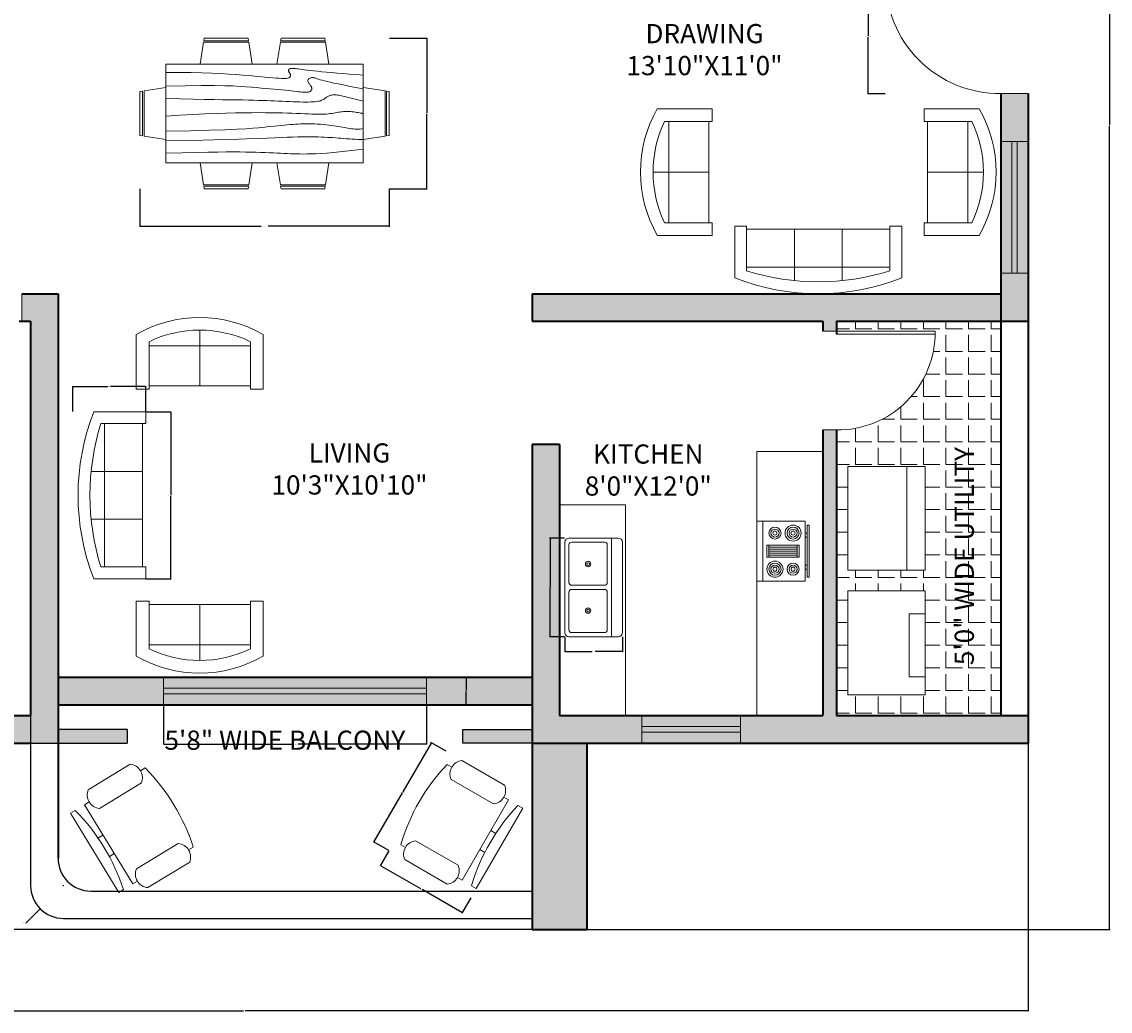
# Model space of a CAD drawing. Units: inches. Extents: x -382 to 250, y 518 to 1732.
# Tile 2 of 8: x -147 to 250, y 518 to 879. Entities that reach past the tile are written whole.
import ezdxf

# ---------------------------------------------------------------- set-up
doc = ezdxf.new("R2010")
doc.units = ezdxf.units.IN
doc.header["$MEASUREMENT"] = 0
for name, color, linetype, lineweight in [('A-ANNO-DIMS', 2, 'Continuous', 18), ('A-AREA-IDEN', 7, 'Continuous', 18), ('A-DOOR', 3, 'Continuous', 18), ('A-EQPM', 9, 'Continuous', 18), ('A-FLOR-CASE', 8, 'Continuous', 18), ('A-FLOR-EDGE', 7, 'Continuous', 25), ('A-FLOR-FIXT', 8, 'Continuous', 18), ('A-FLOR-PATT', 9, 'Continuous', 13), ('A-FURN', 8, 'Continuous', 18), ('A-GLAZ', 4, 'Continuous', 18), ('A-WALL', 7, 'Continuous', 35)]:
    doc.layers.add(name, color=color, linetype=linetype, lineweight=lineweight)
doc.layers.add('A-GLAZ-PATT', color=143, linetype='Continuous', lineweight=13, true_color=0x7aafdf)
doc.layers.add('A-WALL-PATT', color=251, linetype='Continuous', lineweight=13, true_color=0x636466)
doc.styles.get("Standard").update_dxf_attribs({"font": 'arial.ttf'})
doc.dimstyles.get("Standard").update_dxf_attribs({"dimtxt": 0.18, "dimasz": 0.18, "dimexe": 0.18, "dimexo": 0.0625, "dimgap": 0.09, "dimtad": 0, "dimtih": 1, "dimtoh": 1, "dimdec": 4, "dimzin": 0, "dimdsep": 46, "dimtxsty": 'Standard', "dimcen": 0.09, "dimadec": 0, "dimazin": 0, "dimtfac": 1, "dimtdec": 4, "dimtofl": 0, "dimtmove": 0, "dimatfit": 3, "dimfxl": 1, "dimtolj": 1, "dimtzin": 0, "dimarcsym": 0})

# ---------------------------------------------------------------- blocks, each defined once
blk = doc.blocks.new('Dining Set - 36 x 72 in.')
for p, q in [((-22.2343, 26.00059), (-23.4847, 17.99762)), ((-22.2304, 26), (-5.7608, 26)), ((-22, 27.5), (-22.1562, 26.50042)), ((-5.8416, 26.5), (-22.1534, 26.5)), ((-22, 27.5), (-6, 27.5)), ((-5.8437, 26.49966), (-6, 27.5)), ((-4.5152, 17.99762), (-5.7655, 25.99926)), ((5.7657, 26.00059), (4.5153, 17.99762)), ((5.7696, 26), (22.2392, 26)), ((6, 27.5), (5.8438, 26.50042)), ((22.1584, 26.5), (5.8466, 26.5)), ((6, 27.5), (22, 27.5)), ((22.1563, 26.49966), (22, 27.5)), ((23.4848, 17.99762), (22.2345, 25.99926)), ((36, 18), (-36, 18)), ((-36, 18), (-36, -18)), ((36, -18), (36, 18)), ((-45.5, 8), (-44.5004, 8.15617)), ((-45.5, 8), (-45.5, -8)), ((-44.5, -8.15843), (-44.5, 8.15338)), ((-44.0006, 8.23428), (-35.9976, 9.48474)), ((-44, 8.23041), (-44, -8.23915)), ((44.0006, 8.23428), (35.9976, 9.48474)), ((44, 8.23041), (44, -8.23915)), ((44.5, -8.15843), (44.5, 8.15338)), ((45.5, 8), (44.5005, 8.15617)), ((45.5, 8), (45.5, -8)), ((-44.4997, -8.15631), (-45.5, -8)), ((-35.9976, -9.48476), (-43.9993, -8.2345)), ((35.9976, -9.48476), (43.9993, -8.2345)), ((44.4997, -8.15631), (45.5, -8)), ((-36, -18), (36, -18)), ((-22.2343, -26.0006), (-23.4847, -17.99762)), ((-4.5152, -17.99762), (-5.7655, -25.99928)), ((5.7657, -26.0006), (4.5153, -17.99762)), ((23.4848, -17.99762), (22.2345, -25.99928)), ((-22.2304, -26), (-5.7608, -26)), ((-22, -27.5), (-22.1562, -26.50044)), ((-5.8416, -26.5), (-22.1534, -26.5)), ((-22, -27.5), (-6, -27.5)), ((-5.8437, -26.49967), (-6, -27.5)), ((5.7696, -26), (22.2392, -26)), ((6, -27.5), (5.8438, -26.50044)), ((22.1584, -26.5), (5.8466, -26.5)), ((6, -27.5), (22, -27.5)), ((22.1563, -26.49967), (22, -27.5))]:
    blk.add_line(p, q)
for points in [[(-36, 15), (-31.1772, 14.97754), (-26.8079, 14.91406), (-22.8538, 14.81543), (-19.276, 14.6875), (-16.0362, 14.53613), (-13.0957, 14.36718), (-10.4159, 14.18652), (-7.9583, 14), (-5.6904, 13.81315), (-3.6035, 13.63021), (-1.6954, 13.45508), (0.0365, 13.29166), (1.5945, 13.14388), (2.9811, 13.01562), (4.1988, 12.9108), (5.25, 12.83333), (6.1393, 12.78613), (6.8802, 12.76823), (7.4883, 12.77767), (7.9792, 12.8125), (8.3685, 12.87077), (8.6719, 12.95052), (8.9049, 13.0498), (9.0833, 13.16666), (9.2205, 13.29899), (9.3216, 13.44401), (9.3895, 13.59879), (9.4271, 13.76041), (9.4373, 13.92594), (9.4232, 14.09245), (9.3875, 14.257), (9.3333, 14.41666), (9.2638, 14.56917), (9.1836, 14.71484), (9.0975, 14.85465), (9.0104, 14.98958), (8.9272, 15.1206), (8.8529, 15.2487), (8.7922, 15.37483), (8.75, 15.5), (8.7305, 15.62467), (8.7344, 15.74739), (8.7617, 15.86621), (8.8125, 15.97916), (8.8867, 16.08431), (8.9844, 16.17968), (9.1055, 16.26334), (9.25, 16.33333), (9.4189, 16.38802), (9.6172, 16.42708), (9.8506, 16.45052), (10.125, 16.45833), (10.4463, 16.45052), (10.8203, 16.42708), (11.2529, 16.38802), (11.75, 16.33333), (12.3184, 16.26318), (12.9694, 16.17838), (13.7151, 16.07991), (14.5677, 15.96875), (15.5395, 15.84586), (16.6426, 15.71224), (17.8893, 15.56884), (19.2917, 15.41666), (20.859, 15.25667), (22.5879, 15.08984), (24.4721, 14.91715), (26.5052, 14.73958), (28.6809, 14.5581), (30.9929, 14.3737), (33.4347, 14.18733), (36, 14)], [(-36, 10), (-28.9766, 10.14274), (-23.1725, 10.20442), (-18.4241, 10.19775), (-14.5677, 10.13541), (-11.4399, 10.03011), (-8.877, 9.89453), (-6.7154, 9.74137), (-4.7917, 9.58333), (-2.9698, 9.43082), (-1.2246, 9.28515), (0.4415, 9.14534), (2.026, 9.01041), (3.5266, 8.87939), (4.9408, 8.7513), (6.266, 8.62516), (7.5, 8.5), (8.6411, 8.37549), (9.6914, 8.2539), (10.6538, 8.13818), (11.5312, 8.03125), (12.3267, 7.93603), (13.043, 7.85547), (13.6831, 7.79248), (14.25, 7.75), (14.7471, 7.7303), (15.1797, 7.73307), (15.5537, 7.75732), (15.875, 7.80208), (16.1494, 7.86637), (16.3828, 7.94922), (16.5811, 8.04964), (16.75, 8.16666), (16.8944, 8.29915), (17.0143, 8.44531), (17.1089, 8.60319), (17.1771, 8.77083), (17.218, 8.94629), (17.2305, 9.1276), (17.2137, 9.31282), (17.1667, 9.5), (17.0895, 9.6875), (16.987, 9.875), (16.8649, 10.0625), (16.7292, 10.25), (16.5856, 10.4375), (16.4401, 10.625), (16.2985, 10.8125), (16.1667, 11), (16.05, 11.18733), (15.9518, 11.3737), (15.8752, 11.5581), (15.8229, 11.73958), (15.798, 11.91715), (15.8034, 12.08984), (15.842, 12.25667), (15.9167, 12.41666), (16.0295, 12.56836), (16.1784, 12.70833), (16.3605, 12.83268), (16.5729, 12.9375), (16.8127, 13.01888), (17.0768, 13.07291), (17.3625, 13.0957), (17.6667, 13.08333), (17.9894, 13.03312), (18.3418, 12.94726), (18.7382, 12.82918), (19.1927, 12.68229), (19.7195, 12.51001), (20.3327, 12.31575), (21.0465, 12.10294), (21.875, 11.875), (22.8357, 11.63354), (23.959, 11.37304), (25.2786, 11.08618), (26.8282, 10.76562), (28.6414, 10.40405), (30.752, 9.99414), (33.1936, 9.52856), (36, 9)], [(-36, 5.5), (-30.7157, 5.3348), (-26.069, 5.20963), (-21.9946, 5.11767), (-18.4271, 5.05208), (-15.3009, 5.00602), (-12.5508, 4.97265), (-10.1112, 4.94515), (-7.9167, 4.91666), (-5.909, 4.88167), (-4.0586, 4.83984), (-2.3429, 4.79215), (-0.7396, 4.73958), (0.7739, 4.6831), (2.22, 4.6237), (3.6213, 4.56233), (5, 4.5), (6.373, 4.43782), (7.7344, 4.3776), (9.0723, 4.32129), (10.375, 4.27083), (11.6309, 4.22819), (12.8281, 4.19531), (13.9551, 4.17415), (15, 4.16666), (15.954, 4.17448), (16.819, 4.19791), (17.6001, 4.23698), (18.3021, 4.29166), (18.9299, 4.36198), (19.4883, 4.44791), (19.9823, 4.54948), (20.4167, 4.66666), (20.7969, 4.79899), (21.1302, 4.94401), (21.4245, 5.09879), (21.6875, 5.26041), (21.9271, 5.42594), (22.1511, 5.59245), (22.3672, 5.757), (22.5834, 5.91666), (22.8065, 6.06868), (23.0404, 6.21093), (23.2879, 6.34147), (23.5521, 6.45833), (23.8358, 6.55957), (24.142, 6.64323), (24.4735, 6.70735), (24.8334, 6.75), (25.2235, 6.76969), (25.642, 6.76692), (26.0858, 6.74267), (26.5521, 6.69791), (27.0379, 6.63362), (27.5404, 6.55078), (28.0565, 6.45036), (28.5834, 6.33333), (29.1242, 6.19987), (29.7071, 6.04687), (30.3661, 5.87044), (31.1354, 5.66666), (32.0493, 5.43164), (33.142, 5.16146), (34.4475, 4.85221), (36, 4.5)], [(-36, -1), (-30.7915, -0.6591), (-26.0195, -0.38216), (-21.6519, -0.16284), (-17.6563, 0.00521), (-14.0005, 0.12833), (-10.6523, 0.21289), (-7.5796, 0.26522), (-4.75, 0.29166), (-2.134, 0.29793), (0.2878, 0.28711), (2.5317, 0.26163), (4.6146, 0.22396), (6.5529, 0.17651), (8.3633, 0.12174), (10.0623, 0.06209), (11.6667, 0), (13.1899, -0.06201), (14.6341, -0.1211), (15.9982, -0.17432), (17.2813, -0.21875), (18.4823, -0.25147), (19.6003, -0.26953), (20.6343, -0.27002), (21.5834, -0.25), (22.4481, -0.20768), (23.2357, -0.14584), (23.9549, -0.06836), (24.6146, 0.02083), (25.2235, 0.11784), (25.7904, 0.21875), (26.3241, 0.31966), (26.8334, 0.41666), (27.3265, 0.50618), (27.8099, 0.58593), (28.2894, 0.65397), (28.7709, 0.70833), (29.2601, 0.74707), (29.763, 0.76823), (30.2855, 0.76985), (30.8334, 0.75), (31.4088, 0.70784), (31.9994, 0.64713), (32.589, 0.57275), (33.1615, 0.48958), (33.7008, 0.4025), (34.1908, 0.3164), (34.6153, 0.23616), (34.9584, 0.16666), (35.2099, 0.11165), (35.3848, 0.07031), (35.504, 0.04069), (35.5886, 0.02083), (35.6594, 0.00879), (35.7377, 0.0026), (35.8442, 0.00032), (36, 0)], [(-36, -6.5), (-27.1843, -6.31267), (-20.084, -6.1263), (-14.469, -5.9419), (-10.1094, -5.76042), (-6.7752, -5.58285), (-4.2363, -5.41016), (-2.2629, -5.24333), (-0.625, -5.08334), (0.8708, -4.93099), (2.2715, -4.78646), (3.5872, -4.64974), (4.8281, -4.52084), (6.0046, -4.39974), (7.127, -4.28646), (8.2053, -4.18099), (9.25, -4.08334), (10.2705, -3.99382), (11.2734, -3.91407), (12.2647, -3.84603), (13.25, -3.79167), (14.2354, -3.75293), (15.2266, -3.73177), (16.2295, -3.73015), (17.25, -3.75), (18.2912, -3.79248), (19.3451, -3.85547), (20.4009, -3.93604), (21.4479, -4.03125), (22.4754, -4.13819), (23.4727, -4.25391), (24.4289, -4.37549), (25.3334, -4.5), (26.1785, -4.62492), (26.9694, -4.74935), (27.7145, -4.87281), (28.4219, -4.99479), (29.1, -5.11483), (29.7572, -5.23242), (30.4016, -5.34709), (31.0417, -5.45834), (31.6837, -5.56437), (32.3262, -5.65821), (32.9658, -5.73153), (33.599, -5.77604), (34.2224, -5.78345), (34.8327, -5.74545), (35.4264, -5.65373), (36, -5.5)], [(-36, -10), (-26.4022, -9.81299), (-18.4675, -9.62891), (-11.9839, -9.45069), (-6.7396, -9.28125), (-2.5226, -9.12354), (0.8789, -8.98047), (3.6769, -8.85498), (6.0833, -8.75), (8.2767, -8.66765), (10.3021, -8.60677), (12.1712, -8.56543), (13.8958, -8.54167), (15.4876, -8.53353), (16.9583, -8.53907), (18.3197, -8.55632), (19.5834, -8.58334), (20.7616, -8.61841), (21.8685, -8.66081), (22.9188, -8.71004), (23.9271, -8.76563), (24.9081, -8.82707), (25.8763, -8.89388), (26.8465, -8.96558), (27.8334, -9.04167), (28.8474, -9.12118), (29.8828, -9.20117), (30.93, -9.27824), (31.9792, -9.34896), (33.0205, -9.40991), (34.0443, -9.45768), (35.0407, -9.48885), (36, -9.5)], [(-36, -14.5), (-30.0881, -14.33513), (-25.0332, -14.21224), (-20.7312, -14.12647), (-17.0781, -14.07292), (-13.97, -14.04671), (-11.3027, -14.04297), (-8.9724, -14.05681), (-6.875, -14.08334), (-4.9224, -14.11833), (-3.0905, -14.16016), (-1.3709, -14.20785), (0.2448, -14.26042), (1.7647, -14.3169), (3.1973, -14.3763), (4.5507, -14.43767), (5.8333, -14.5), (7.0554, -14.5621), (8.235, -14.62175), (9.3922, -14.67652), (10.5469, -14.72396), (11.7192, -14.76164), (12.929, -14.78711), (14.1965, -14.79794), (15.5417, -14.79167), (16.9933, -14.76424), (18.6152, -14.70508), (20.4804, -14.60197), (22.6615, -14.44271), (25.2312, -14.21509), (28.2624, -13.9069), (31.8277, -13.50594), (36, -13)]]:
    blk.add_lwpolyline(points)
blk = doc.blocks.new('Chair - Desk')
for p, q in [((-8.5, 0), (-8.5, -1)), ((-8.5, 0), (8.5, 0)), ((8.5, 0), (8.5, -1)), ((-2, -3), (-2, -1.9355)), ((2, -1.9576), (2, -3)), ((-8.5, -3), (-8.5, -4)), ((-8.5, -3), (8.5, -3)), ((8.5, -3), (8.5, -4)), ((-10.5, -5), (-10.5, -14)), ((-6.5, -14), (-6.5, -5)), ((6.5, -5), (6.5, -14)), ((10.5, -14), (10.5, -5)), ((-8.5, -15), (-8.5, -16)), ((8.5, -15), (8.5, -16))]:
    blk.add_line(p, q)
for centre, radius, start, end in [((0, 34.625), 36.625, 256.5803, 283.4197), ((-8.5, -6.5), 2.5, 36.8699, 143.1301), ((8.5, -6.5), 2.5, 36.8699, 143.1301), ((-8.5, -12.5), 2.5, 216.8699, 323.1301), ((8.5, -12.5), 2.5, 216.8699, 323.1301), ((0, 19.625), 36.625, 256.5803, 283.4197)]:
    blk.add_arc(centre, radius, start, end)
blk = doc.blocks.new('Sofa - Roundback 7 ft.')
for p, q in [((-12.00002, -32.4421), (-12.00003, -6.5971)), ((11.99997, -32.4421), (11.99998, -6.5971)), ((-36.000027, -34), (-36.000027, -11.4696)), ((-35.999844, -13.3819), (35.9998, -13.3819)), ((35.99998, -34), (35.99998, -11.4696)), ((-36.000027, -32.4421), (35.99998, -32.4421))]:
    blk.add_line(p, q)
for points in [[(-36.000027, -34), (-42.000027, -34), (-42.000027, -8)], [(41.99998, -8), (41.99998, -34), (35.99998, -34)]]:
    blk.add_lwpolyline(points)
for centre, radius, start, end in [((0, -114.25), 114.25, 68.43141, 111.5686), ((-0.00001, -127.1968), 121.1968, 72.72033, 107.2797)]:
    blk.add_arc(centre, radius, start, end)
blk = doc.blocks.new('Sofa - Roundback Loveseat 5 ft.')
for p, q in [((0, -32.44198), (0, -5.99998)), ((-24, -33.99998), (-24, -11.46958)), ((-23.9998, -13.38178), (23.99986, -13.38178)), ((24.00004, -33.99998), (24.00004, -11.46958)), ((-24, -32.44198), (24.00004, -32.44198))]:
    blk.add_line(p, q)
for points in [[(-24, -33.99998), (-30, -33.99998), (-30, -7.99998)], [(30.00004, -7.99998), (30.00004, -33.99998), (24.00004, -33.99998)]]:
    blk.add_lwpolyline(points)
for centre, radius, start, end in [((0, -60.24998), 60.24998, 60.13715, 119.8628), ((0, -61.38438), 55.38444, 64.32083, 115.6792)]:
    blk.add_arc(centre, radius, start, end)
blk = doc.blocks.new('Sink-double - 36 in top')
for p, q in [((-18, -4), (18, -4)), ((-0.75, -18.5), (-0.75, -6.5)), ((0.75, -6.5), (0.75, -18.5))]:
    blk.add_line(p, q)
for points in [[(-16.5, 0), (16.5, 0)], [(-18, -19.5), (-18, -1.5)], [(18, -1.5), (18, -19.5)], [(-16.5, -18.5), (-16.5, -6.5)], [(-15.5, -5.5), (-1.75, -5.5)], [(1.75, -5.5), (15.5, -5.5)], [(16.5, -6.5), (16.5, -18.5)], [(-1.75, -19.5), (-15.5, -19.5)], [(15.5, -19.5), (1.75, -19.5)], [(16.5, -21), (-16.5, -21)]]:
    blk.add_lwpolyline(points)
for centre, radius in [((-8.5, -12.5), 1), ((8.5, -12.5), 1), ((-8.5, -12.5), 0.5), ((8.5, -12.5), 0.5)]:
    blk.add_circle(centre, radius)
for centre, radius, start, end in [((-16.5, -1.5), 1.5, 90, 180), ((16.5, -1.5), 1.5, 0, 90), ((-15.5, -6.5), 1, 90, 180), ((-1.75, -6.5), 1, 0, 90), ((1.75, -6.5), 1, 90, 180), ((15.5, -6.5), 1, 0, 90), ((-16.5, -19.5), 1.5, 180, 270), ((-15.5, -18.5), 1, 180, 270), ((-1.75, -18.5), 1, 270, 0), ((1.75, -18.5), 1, 180, 270), ((15.5, -18.5), 1, 270, 0), ((16.5, -19.5), 1.5, 270, 0)]:
    blk.add_arc(centre, radius, start, end)
blk = doc.blocks.new('Range-Oven - 30 in top')
for p, q in [((0, -3), (30, -3)), ((12, -6), (18, -6)), ((13, -20), (13, -6)), ((14, -6), (14, -20)), ((15, -20), (15, -6)), ((16, -6), (16, -20)), ((17, -20), (17, -6)), ((18, -20), (12, -20)), ((6, -24), (6, -25)), ((8, -25), (8, -24)), ((22, -25), (22, -24)), ((24, -24), (24, -25))]:
    blk.add_line(p, q)
for points in [[(0, -24), (0, 0), (30, 0), (30, -24)], [(12, -21), (12, -5), (18, -5), (18, -21)], [(2, -26), (2, -25), (28, -25), (28, -26)]]:
    blk.add_lwpolyline(points, close=True)
for centre, radius in [((6, -9), 4), ((6, -9), 3), ((6, -9), 2), ((6, -9), 1), ((24, -9), 3), ((24, -9), 2), ((24, -9), 1), ((6, -18), 3), ((6, -18), 2), ((24, -18), 4), ((24, -18), 3), ((24, -18), 2), ((6, -18), 1), ((24, -18), 1)]:
    blk.add_circle(centre, radius)
blk = doc.blocks.new('DOOR-SWING-36IN')
for p, q in [((-1, 0), (-1, 36)), ((0, 0), (0, 36))]:
    blk.add_line(p, q)
blk.add_arc((-0.5, 0.5), 35.5, 89.1931, 180.8069)
blk = doc.blocks.new('GLAZ-BALCONY-96IN')
for p, q in [((0, 10), (0, 0)), ((96, 10), (96, 0)), ((0, 6), (96, 6)), ((0, 4), (96, 4))]:
    blk.add_line(p, q)
blk = doc.blocks.new('DOOR-ENTRY-42IN')
for p, q in [((0, 0), (-42, 0)), ((0, -1), (-42, -1))]:
    blk.add_line(p, q)
blk.add_arc((-0.5, -0.5), 41.5, 179.3097, 270.6903)
blk = doc.blocks.new('*D34')
at = {"layer": 'A-ANNO-DIMS', "color": 0, "lineweight": -2, "transparency": 16777216}
for p, q in [((-102.16, 736.99), (-92.9, 736.99)), ((-93.08, 736.81), (-93.08, 706.68)), ((-93.08, 676.19), (-93.08, 706.32)), ((-102.16, 676.01), (-92.9, 676.01))]:
    blk.add_line(p, q, dxfattribs=at)
at = {"layer": 'A-ANNO-DIMS', "color": 0, "transparency": 16777216}
for points in [[(-93.11, 736.81), (-93.05, 736.81), (-93.08, 736.99)], [(-93.11, 676.19), (-93.05, 676.19), (-93.08, 676.01)]]:
    blk.add_solid(points, dxfattribs=at)
at = {"layer": 'Defpoints', "color": 0, "transparency": 16777216}
for p in [(-102.23, 736.99), (-93.08, 736.99), (-102.23, 676.01)]:
    blk.add_point(p, dxfattribs=at)
at = {"layer": 'A-ANNO-DIMS', "color": 0, "transparency": 16777216, "insert": (-93.08, 706.5), "char_height": 0.18, "attachment_point": 5}
blk.add_mtext('\\A1;SOFA 61 TYP.', dxfattribs=at)
blk = doc.blocks.new('*D35')
at = {"layer": 'A-ANNO-DIMS', "color": 0, "lineweight": -2, "transparency": 16777216}
for p, q in [((-128.84, 737.05), (-128.84, 746.32)), ((-128.66, 746.14), (-116.06, 746.14)), ((-102.41, 746.14), (-115.01, 746.14)), ((-102.23, 737.05), (-102.23, 746.32))]:
    blk.add_line(p, q, dxfattribs=at)
at = {"layer": 'A-ANNO-DIMS', "color": 0, "transparency": 16777216}
for points in [[(-128.66, 746.17), (-128.66, 746.11), (-128.84, 746.14)], [(-102.41, 746.17), (-102.41, 746.11), (-102.23, 746.14)]]:
    blk.add_solid(points, dxfattribs=at)
at = {"layer": 'Defpoints', "color": 0, "transparency": 16777216}
for p in [(-128.84, 746.14), (-128.84, 736.99), (-102.23, 736.99)]:
    blk.add_point(p, dxfattribs=at)
at = {"layer": 'A-ANNO-DIMS', "color": 0, "transparency": 16777216, "insert": (-115.54, 746.14), "char_height": 0.18, "attachment_point": 5}
blk.add_mtext('\\A1;27 TYP.', dxfattribs=at)
blk = doc.blocks.new('*D36')
at = {"layer": 'A-ANNO-DIMS', "color": 0, "lineweight": -2, "transparency": 16777216}
for p, q in [((1.91, 616.01), (-8.35, 598.25)), ((7.37, 613.06), (1.84, 616.26)), ((-18.82, 580.12), (-8.56, 597.88)), ((-13.53, 576.86), (-19.06, 580.05))]:
    blk.add_line(p, q, dxfattribs=at)
at = {"layer": 'A-ANNO-DIMS', "color": 0, "transparency": 16777216}
for points in [[(1.88, 616.02), (1.93, 615.99), (2, 616.17)], [(-18.84, 580.13), (-18.79, 580.1), (-18.91, 579.96)]]:
    blk.add_solid(points, dxfattribs=at)
at = {"layer": 'Defpoints', "color": 0, "transparency": 16777216}
for p in [(7.43, 613.03), (-18.91, 579.96), (-13.48, 576.83)]:
    blk.add_point(p, dxfattribs=at)
at = {"layer": 'A-ANNO-DIMS', "color": 0, "transparency": 16777216, "insert": (-8.46, 598.06), "char_height": 0.18, "attachment_point": 5}
blk.add_mtext('\\A1;CHAIR 42 TYP.', dxfattribs=at)
blk = doc.blocks.new('*D37')
at = {"layer": 'A-ANNO-DIMS', "color": 0, "lineweight": -2, "transparency": 16777216}
for p, q in [((-13.51, 576.77), (-16.7, 571.24)), ((-16.46, 571.31), (-1.99, 562.95)), ((13.12, 554.23), (-1.36, 562.59)), ((16.38, 559.52), (13.18, 553.99))]:
    blk.add_line(p, q, dxfattribs=at)
at = {"layer": 'A-ANNO-DIMS', "color": 0, "transparency": 16777216}
for points in [[(-16.44, 571.33), (-16.47, 571.28), (-16.61, 571.4)], [(13.13, 554.26), (13.1, 554.21), (13.27, 554.14)]]:
    blk.add_solid(points, dxfattribs=at)
at = {"layer": 'Defpoints', "color": 0, "transparency": 16777216}
for p in [(-13.48, 576.83), (16.41, 559.57), (13.27, 554.14)]:
    blk.add_point(p, dxfattribs=at)
at = {"layer": 'A-ANNO-DIMS', "color": 0, "transparency": 16777216, "insert": (-1.67, 562.77), "char_height": 0.18, "attachment_point": 5}
blk.add_mtext('\\A1;35 TYP.', dxfattribs=at)
blk = doc.blocks.new('*D40')
at = {"layer": 'A-ANNO-DIMS', "color": 0, "lineweight": -2, "transparency": 16777216}
for p, q in [((-104.34, 818.28), (-104.34, 804.52)), ((-13.34, 818.28), (-13.34, 804.52)), ((-104.16, 804.7), (-60.12, 804.7)), ((-13.52, 804.7), (-57.56, 804.7))]:
    blk.add_line(p, q, dxfattribs=at)
at = {"layer": 'A-ANNO-DIMS', "color": 0, "transparency": 16777216}
for points in [[(-104.16, 804.73), (-104.16, 804.67), (-104.34, 804.7)], [(-13.52, 804.73), (-13.52, 804.67), (-13.34, 804.7)]]:
    blk.add_solid(points, dxfattribs=at)
at = {"layer": 'Defpoints', "color": 0, "transparency": 16777216}
for p in [(-104.34, 818.35), (-13.34, 818.35), (-13.34, 804.7)]:
    blk.add_point(p, dxfattribs=at)
at = {"layer": 'A-ANNO-DIMS', "color": 0, "transparency": 16777216, "insert": (-58.84, 804.7), "char_height": 0.18, "attachment_point": 5}
blk.add_mtext('\\A1;DINING SET 91 TYP.', dxfattribs=at)
blk = doc.blocks.new('*D41')
at = {"layer": 'A-ANNO-DIMS', "color": 0, "lineweight": -2, "transparency": 16777216}
for p, q in [((-13.28, 873.35), (0.49, 873.35)), ((0.31, 873.17), (0.31, 846.03)), ((0.31, 818.53), (0.31, 845.66)), ((-13.28, 818.35), (0.49, 818.35))]:
    blk.add_line(p, q, dxfattribs=at)
at = {"layer": 'A-ANNO-DIMS', "color": 0, "transparency": 16777216}
for points in [[(0.28, 873.17), (0.34, 873.17), (0.31, 873.35)], [(0.28, 818.53), (0.34, 818.53), (0.31, 818.35)]]:
    blk.add_solid(points, dxfattribs=at)
at = {"layer": 'Defpoints', "color": 0, "transparency": 16777216}
for p in [(-13.34, 873.35), (0.31, 873.35), (-13.34, 818.35)]:
    blk.add_point(p, dxfattribs=at)
at = {"layer": 'A-ANNO-DIMS', "color": 0, "transparency": 16777216, "insert": (0.31, 845.85), "char_height": 0.18, "attachment_point": 5}
blk.add_mtext('\\A1;55 TYP.', dxfattribs=at)
blk = doc.blocks.new('*D46')
at = {"layer": 'A-ANNO-DIMS', "color": 0, "lineweight": -2, "transparency": 16777216}
for p, q in [((50.64, 690.89), (45.12, 690.89)), ((45.3, 690.71), (45.3, 673.08)), ((45.3, 655.07), (45.3, 672.71)), ((50.64, 654.89), (45.12, 654.89))]:
    blk.add_line(p, q, dxfattribs=at)
at = {"layer": 'A-ANNO-DIMS', "color": 0, "transparency": 16777216}
for points in [[(45.27, 690.71), (45.33, 690.71), (45.3, 690.89)], [(45.27, 655.07), (45.33, 655.07), (45.3, 654.89)]]:
    blk.add_solid(points, dxfattribs=at)
at = {"layer": 'Defpoints', "color": 0, "transparency": 16777216}
for p in [(50.7, 690.89), (45.3, 654.89), (50.7, 654.89)]:
    blk.add_point(p, dxfattribs=at)
at = {"layer": 'A-ANNO-DIMS', "color": 0, "transparency": 16777216, "insert": (45.3, 672.89), "char_height": 0.18, "attachment_point": 5}
blk.add_mtext('\\A1;SINK 36 TYP.', dxfattribs=at)
blk = doc.blocks.new('*D47')
at = {"layer": 'A-ANNO-DIMS', "color": 0, "lineweight": -2, "transparency": 16777216}
for p, q in [((50.7, 654.83), (50.7, 649.31)), ((71.7, 654.83), (71.7, 649.31)), ((50.88, 649.49), (60.67, 649.49)), ((71.52, 649.49), (61.73, 649.49))]:
    blk.add_line(p, q, dxfattribs=at)
at = {"layer": 'A-ANNO-DIMS', "color": 0, "transparency": 16777216}
for points in [[(50.88, 649.52), (50.88, 649.46), (50.7, 649.49)], [(71.52, 649.52), (71.52, 649.46), (71.7, 649.49)]]:
    blk.add_solid(points, dxfattribs=at)
at = {"layer": 'Defpoints', "color": 0, "transparency": 16777216}
for p in [(50.7, 654.89), (71.7, 654.89), (71.7, 649.49)]:
    blk.add_point(p, dxfattribs=at)
at = {"layer": 'A-ANNO-DIMS', "color": 0, "transparency": 16777216, "insert": (61.2, 649.49), "char_height": 0.18, "attachment_point": 5}
blk.add_mtext('\\A1;21 TYP.', dxfattribs=at)
blk = doc.blocks.new('*D58')
at = {"layer": 'A-ANNO-DIMS', "color": 0, "lineweight": -2, "transparency": 16777216}
for p, q in [((167.59, 895.12), (161.15, 895.12)), ((161.33, 894.94), (161.33, 874.24)), ((161.33, 853.17), (161.33, 873.87)), ((167.59, 852.99), (161.15, 852.99))]:
    blk.add_line(p, q, dxfattribs=at)
at = {"layer": 'A-ANNO-DIMS', "color": 0, "transparency": 16777216}
for points in [[(161.3, 894.94), (161.36, 894.94), (161.33, 895.12)], [(161.3, 853.17), (161.36, 853.17), (161.33, 852.99)]]:
    blk.add_solid(points, dxfattribs=at)
at = {"layer": 'Defpoints', "color": 0, "transparency": 16777216}
for p in [(161.33, 895.12), (167.65, 895.12), (167.65, 852.99)]:
    blk.add_point(p, dxfattribs=at)
at = {"layer": 'A-ANNO-DIMS', "color": 0, "transparency": 16777216, "insert": (161.33, 874.06), "char_height": 0.18, "attachment_point": 5}
blk.add_mtext('\\A1;ENTRY DOOR 42 TYP.', dxfattribs=at)
blk = doc.blocks.new('*D66')
at = {"layer": 'A-ANNO-DIMS', "color": 0, "lineweight": -2, "transparency": 16777216}
for p, q in [((-95.72, 630.01), (-95.72, 615.49)), ((0.28, 630.01), (0.28, 615.49)), ((-95.54, 615.67), (-48.83, 615.67)), ((0.1, 615.67), (-46.6, 615.67))]:
    blk.add_line(p, q, dxfattribs=at)
at = {"layer": 'A-ANNO-DIMS', "color": 0, "transparency": 16777216}
for points in [[(-95.54, 615.7), (-95.54, 615.64), (-95.72, 615.67)], [(0.1, 615.7), (0.1, 615.64), (0.28, 615.67)]]:
    blk.add_solid(points, dxfattribs=at)
at = {"layer": 'Defpoints', "color": 0, "transparency": 16777216}
for p in [(-95.72, 630.07), (0.28, 630.07), (0.28, 615.67)]:
    blk.add_point(p, dxfattribs=at)
at = {"layer": 'A-ANNO-DIMS', "color": 0, "transparency": 16777216, "insert": (-47.72, 615.67), "char_height": 0.18, "attachment_point": 5}
blk.add_mtext('\\A1;GLAZING 96 TYP.', dxfattribs=at)
blk = doc.blocks.new('*D67')
at = {"layer": 'A-ANNO-DIMS', "color": 0, "lineweight": -2, "transparency": 16777216}
for p, q in [((0.35, 640.07), (14.86, 640.07)), ((14.68, 639.89), (14.68, 635.25)), ((14.68, 630.25), (14.68, 634.89)), ((0.35, 630.07), (14.86, 630.07))]:
    blk.add_line(p, q, dxfattribs=at)
at = {"layer": 'A-ANNO-DIMS', "color": 0, "transparency": 16777216}
for points in [[(14.65, 639.89), (14.71, 639.89), (14.68, 640.07)], [(14.65, 630.25), (14.71, 630.25), (14.68, 630.07)]]:
    blk.add_solid(points, dxfattribs=at)
at = {"layer": 'Defpoints', "color": 0, "transparency": 16777216}
for p in [(0.28, 640.07), (14.68, 640.07), (0.28, 630.07)]:
    blk.add_point(p, dxfattribs=at)
at = {"layer": 'A-ANNO-DIMS', "color": 0, "transparency": 16777216, "insert": (14.68, 635.07), "char_height": 0.18, "attachment_point": 5}
blk.add_mtext('\\A1;10 TYP.', dxfattribs=at)
blk = doc.blocks.new('*D74')
at = {"layer": 'A-ANNO-DIMS', "color": 0, "lineweight": -2, "transparency": 16777216}
for p, q in [((-352.22, 770.01), (-352.22, 518.19)), ((219.78, 616.01), (219.78, 518.19)), ((-352.04, 518.37), (-66.5, 518.37)), ((219.6, 518.37), (-65.93, 518.37))]:
    blk.add_line(p, q, dxfattribs=at)
at = {"layer": 'A-ANNO-DIMS', "color": 0, "transparency": 16777216}
for points in [[(-352.04, 518.4), (-352.04, 518.34), (-352.22, 518.37)], [(219.6, 518.4), (219.6, 518.34), (219.78, 518.37)]]:
    blk.add_solid(points, dxfattribs=at)
at = {"layer": 'Defpoints', "color": 0, "transparency": 16777216}
for p in [(-352.22, 770.07), (219.78, 616.07), (219.78, 518.37)]:
    blk.add_point(p, dxfattribs=at)
at = {"layer": 'A-ANNO-DIMS', "color": 0, "transparency": 16777216, "insert": (-66.22, 518.37), "char_height": 0.18, "attachment_point": 5}
blk.add_mtext('\\A1;572', dxfattribs=at)
blk = doc.blocks.new('*D75')
at = {"layer": 'A-ANNO-DIMS', "color": 0, "lineweight": -2, "transparency": 16777216}
for p, q in [((77.85, 1135.07), (249.66, 1135.07)), ((249.48, 1134.89), (249.48, 841.75)), ((249.48, 548.25), (249.48, 841.39)), ((58.85, 548.07), (249.66, 548.07))]:
    blk.add_line(p, q, dxfattribs=at)
at = {"layer": 'A-ANNO-DIMS', "color": 0, "transparency": 16777216}
for points in [[(249.45, 1134.89), (249.51, 1134.89), (249.48, 1135.07)], [(249.45, 548.25), (249.51, 548.25), (249.48, 548.07)]]:
    blk.add_solid(points, dxfattribs=at)
at = {"layer": 'Defpoints', "color": 0, "transparency": 16777216}
for p in [(77.78, 1135.07), (249.48, 1135.07), (58.78, 548.07)]:
    blk.add_point(p, dxfattribs=at)
at = {"layer": 'A-ANNO-DIMS', "color": 0, "transparency": 16777216, "insert": (249.48, 841.57), "char_height": 0.18, "attachment_point": 5}
blk.add_mtext('\\A1;587', dxfattribs=at)
blk = doc.blocks.new('*D82')
at = {"layer": 'A-ANNO-DIMS', "color": 0, "lineweight": -2, "transparency": 16777216}
for p, q in [((-298.28, 616.07), (-382.1, 616.07)), ((-381.92, 615.89), (-381.92, 582.25)), ((-381.92, 548.25), (-381.92, 581.89)), ((38.72, 548.07), (-382.1, 548.07))]:
    blk.add_line(p, q, dxfattribs=at)
at = {"layer": 'A-ANNO-DIMS', "color": 0, "transparency": 16777216}
for points in [[(-381.95, 615.89), (-381.89, 615.89), (-381.92, 616.07)], [(-381.95, 548.25), (-381.89, 548.25), (-381.92, 548.07)]]:
    blk.add_solid(points, dxfattribs=at)
at = {"layer": 'Defpoints', "color": 0, "transparency": 16777216}
for p in [(-381.92, 616.07), (-298.22, 616.07), (38.78, 548.07)]:
    blk.add_point(p, dxfattribs=at)
at = {"layer": 'A-ANNO-DIMS', "color": 0, "transparency": 16777216, "insert": (-381.92, 582.07), "char_height": 0.18, "attachment_point": 5}
blk.add_mtext('\\A1;68', dxfattribs=at)
blk = doc.blocks.new('*D97')
at = {"layer": 'A-ANNO-DIMS', "color": 0, "lineweight": -2, "transparency": 16777216}
for p, q in [((-132.31, 564.07), (-132.13, 564.07)), ((-132.22, 563.98), (-132.22, 564.16)), ((-145.79, 550.49), (-140.83, 555.46)), ((-145.97, 550.49), (-145.79, 550.49))]:
    blk.add_line(p, q, dxfattribs=at)
at = {"layer": 'A-ANNO-DIMS', "color": 0, "transparency": 16777216}
blk.add_solid([(-140.85, 555.48), (-140.81, 555.43), (-140.7, 555.58)], dxfattribs=at)
at = {"layer": 'Defpoints', "color": 0, "transparency": 16777216}
for p in [(-132.22, 564.07), (-140.7, 555.58)]:
    blk.add_point(p, dxfattribs=at)
at = {"layer": 'A-ANNO-DIMS', "color": 0, "transparency": 16777216, "insert": (-146.47, 550.49), "char_height": 0.18, "attachment_point": 5}
blk.add_mtext('\\A1;2X R12', dxfattribs=at)

msp = doc.modelspace()

# ---------------------------------------------------------------- hatches: boundary and pattern name
at = {"layer": 'A-FLOR-PATT'}
h = msp.add_hatch(dxfattribs=at)
h.set_pattern_fill('ANGLE', color=256, scale=30)
h.set_pattern_definition([(0, (0, 0), (0, 8.25), [6, -2.25]), (90, (0, 0), (-8.25, 5e-16), [6, -2.25])])
h.paths.add_polyline_path([(149.785, 730.3412), (149.785, 626.0687), (209.785, 626.0687), (209.785, 770.0687), (149.785, 770.0687), (149.785, 766.3412), (185.785, 766.3412, -0.4224878)])
h.paths.add_polyline_path([(182.2198, 717.0512), (182.2198, 679.1922), (175.5093, 679.1922), (153.9541, 679.1922), (153.9541, 717.0512)], flags=16)
h.paths.add_polyline_path([(182.2198, 671.5751), (182.2198, 633.7161), (153.9541, 633.7161), (153.9541, 671.5751)], flags=16)
h.paths.add_polyline_path([(182.2198, 663.2888), (182.2198, 640.2274), (176.3316, 640.2274), (176.3316, 663.2888)], flags=0)
h.paths.add_polyline_path([(203.7907, 640.5939), (203.7907, 727.6785), (189.3657, 727.6785), (189.3657, 640.5939)], flags=24)
at = {"layer": 'A-GLAZ-PATT'}
h = msp.add_hatch(color=256, dxfattribs=at)
h.dxf.hatch_style = 1
h.paths.add_polyline_path([(213.785, 835.596), (209.785, 835.596), (209.785, 787.596), (213.785, 787.596)])
h = msp.add_hatch(color=256, dxfattribs=at)
h.dxf.hatch_style = 1
h.paths.add_polyline_path([(215.785, 835.596), (213.785, 835.596), (213.785, 787.596), (215.785, 787.596)])
h = msp.add_hatch(color=256, dxfattribs=at)
h.dxf.hatch_style = 1
h.paths.add_polyline_path([(219.785, 835.596), (215.785, 835.596), (215.785, 787.596), (219.785, 787.596)])
h = msp.add_hatch(color=256, dxfattribs=at)
h.dxf.hatch_style = 1
h.paths.add_polyline_path([(0.285, 640.0687), (-95.715, 640.0687), (-95.715, 636.0687), (0.285, 636.0687)])
h = msp.add_hatch(color=256, dxfattribs=at)
h.dxf.hatch_style = 1
h.paths.add_polyline_path([(0.285, 636.0687), (-95.715, 636.0687), (-95.715, 634.0687), (0.285, 634.0687)])
h = msp.add_hatch(color=256, dxfattribs=at)
h.dxf.hatch_style = 1
h.paths.add_polyline_path([(0.285, 634.0687), (-95.715, 634.0687), (-95.715, 630.0687), (0.285, 630.0687)])
h = msp.add_hatch(color=256, dxfattribs=at)
h.dxf.hatch_style = 1
h.paths.add_polyline_path([(114.785, 626.0687), (78.785, 626.0687), (78.785, 622.0687), (114.785, 622.0687)])
h = msp.add_hatch(color=256, dxfattribs=at)
h.dxf.hatch_style = 1
h.paths.add_polyline_path([(114.785, 622.0687), (78.785, 622.0687), (78.785, 620.0687), (114.785, 620.0687)])
h = msp.add_hatch(color=256, dxfattribs=at)
h.dxf.hatch_style = 1
h.paths.add_polyline_path([(114.785, 620.0687), (78.785, 620.0687), (78.785, 616.0687), (114.785, 616.0687)])
at = {"layer": 'A-WALL-PATT'}
h = msp.add_hatch(color=256, dxfattribs=at)
h.dxf.hatch_style = 1
h.paths.add_polyline_path([(219.785, 853.1233), (209.785, 853.1233), (209.785, 835.596), (219.785, 835.596)])
h = msp.add_hatch(color=256, dxfattribs=at)
h.dxf.hatch_style = 1
h.paths.add_polyline_path([(219.785, 787.596), (209.785, 787.596), (209.785, 770.0687), (219.785, 770.0687), (219.785, 771.0687)])
h = msp.add_hatch(color=256, dxfattribs=at)
h.dxf.hatch_style = 1
h.paths.add_polyline_path([(-134.215, 780.0687), (-147.4355, 780.0687), (-147.4355, 770.0687), (-144.215, 770.0687), (-144.215, 626.0687), (-144.215, 616.0687), (-134.215, 616.0687)])
h = msp.add_hatch(color=256, dxfattribs=at)
h.dxf.hatch_style = 1
h.paths.add_polyline_path([(209.785, 780.0687), (38.785, 780.0687), (38.785, 770.0687), (144.785, 770.0687), (144.785, 766.3412), (149.785, 766.3412), (149.785, 770.0687), (209.785, 770.0687)])
h = msp.add_hatch(color=256, dxfattribs=at)
h.dxf.hatch_style = 1
h.paths.add_polyline_path([(219.785, 626.0687), (149.785, 626.0687), (149.785, 730.3412), (144.785, 730.3412), (144.785, 626.0687), (114.785, 626.0687), (114.785, 616.0687), (219.785, 616.0687)])
h = msp.add_hatch(color=256, dxfattribs=at)
h.dxf.hatch_style = 1
h.paths.add_polyline_path([(48.785, 724.9709), (38.785, 724.9709), (38.785, 616.0687), (78.785, 616.0687), (78.785, 626.0687), (48.785, 626.0687)])
h = msp.add_hatch(color=256, dxfattribs=at)
h.dxf.hatch_style = 1
h.paths.add_polyline_path([(-95.715, 640.0687), (-134.215, 640.0687), (-134.215, 630.0687), (-95.715, 630.0687)])
h = msp.add_hatch(color=256, dxfattribs=at)
h.dxf.hatch_style = 1
h.paths.add_polyline_path([(38.785, 640.0687), (0.285, 640.0687), (0.285, 630.0687), (38.785, 630.0687)])
h = msp.add_hatch(color=256, dxfattribs=at)
h.dxf.hatch_style = 1
h.paths.add_polyline_path([(-144.215, 626.0687), (-194.615, 626.0687), (-194.615, 616.0687), (-144.215, 616.0687)])
h = msp.add_hatch(color=256, dxfattribs=at)
h.dxf.hatch_style = 1
h.paths.add_polyline_path([(-108.9736, 621.0687), (-134.215, 621.0687), (-134.215, 616.0687), (-108.9736, 616.0687)])
h = msp.add_hatch(color=256, dxfattribs=at)
h.dxf.hatch_style = 1
h.paths.add_polyline_path([(38.785, 621.0687), (13.5435, 621.0687), (13.5435, 616.0687), (38.785, 616.0687)])
h = msp.add_hatch(color=256, dxfattribs=at)
h.dxf.hatch_style = 1
h.paths.add_polyline_path([(58.785, 616.0687), (38.785, 616.0687), (38.785, 548.0687), (58.785, 548.0687)])

# ---------------------------------------------------------------- linework, layer by layer
at = {"layer": 'A-DOOR'}
for p, q in [((209.785, 853.1233), (219.785, 853.1233)), ((-147.4355, 770.0687), (-147.4355, 780.0687)), ((149.785, 766.3412), (144.785, 766.3412)), ((149.785, 730.3412), (144.785, 730.3412))]:
    msp.add_line(p, q, dxfattribs=at)
at = {"layer": 'A-EQPM'}
for points in [[(153.9541, 679.1922), (182.2198, 679.1922), (182.2198, 717.0512), (153.9541, 717.0512)], [(182.2198, 717.0512), (175.5093, 717.0512), (175.5093, 679.1922), (182.2198, 679.1922)], [(153.9541, 633.7161), (182.2198, 633.7161), (182.2198, 671.5751), (153.9541, 671.5751)], [(182.2198, 663.2888), (176.3316, 663.2888), (176.3316, 640.2274), (182.2198, 640.2274)]]:
    msp.add_lwpolyline(points, close=True, dxfattribs=at)
at = {"layer": 'A-FLOR-CASE'}
for p, q in [((120.785, 722.5328), (120.785, 626.0687)), ((120.785, 722.5328), (144.785, 722.5328)), ((48.785, 703.0687), (72.785, 703.0687)), ((72.785, 703.0687), (72.785, 626.0687))]:
    msp.add_line(p, q, dxfattribs=at)
at = {"layer": 'A-FLOR-EDGE'}
for p, q in [((-144.215, 626.0687), (-144.215, 564.0687)), ((-108.9736, 621.0687), (-134.215, 621.0687)), ((-108.9736, 621.0687), (-108.9736, 616.0687)), ((13.5435, 616.0687), (13.5435, 621.0687)), ((13.5435, 621.0687), (38.785, 621.0687)), ((-144.215, 616.0687), (-108.9736, 616.0687)), ((38.785, 616.0687), (13.5435, 616.0687)), ((-122.215, 562.0687), (38.785, 562.0687)), ((-132.215, 552.0687), (38.785, 552.0687))]:
    msp.add_line(p, q, dxfattribs=at)
for centre in [(-122.215, 574.0687), (-132.215, 564.0687)]:
    msp.add_arc(centre, 12, 180, 270, dxfattribs=at)
at = {"layer": 'A-GLAZ'}
for p, q in [((209.785, 835.596), (219.785, 835.596)), ((213.785, 835.596), (213.785, 787.596)), ((215.785, 835.596), (215.785, 787.596)), ((209.785, 787.596), (219.785, 787.596)), ((78.785, 626.0687), (78.785, 616.0687)), ((114.785, 626.0687), (114.785, 616.0687)), ((78.785, 622.0687), (114.785, 622.0687)), ((78.785, 620.0687), (114.785, 620.0687))]:
    msp.add_line(p, q, dxfattribs=at)
at = {"layer": 'A-WALL'}
for p, q in [((209.785, 853.1233), (209.785, 770.0687)), ((219.785, 853.1233), (219.785, 771.0687)), ((-147.4355, 780.0687), (-134.215, 780.0687)), ((-134.215, 780.0687), (-134.215, 574.0687)), ((38.785, 780.0687), (38.785, 770.0687)), ((38.785, 780.0687), (209.785, 780.0687)), ((219.785, 771.0687), (219.785, 616.0687)), ((-148.4355, 770.0687), (-144.215, 770.0687)), ((-144.215, 770.0687), (-144.215, 626.0687)), ((38.785, 770.0687), (144.785, 770.0687)), ((144.785, 770.0687), (144.785, 766.3412)), ((149.785, 770.0687), (149.785, 765.3412)), ((149.785, 770.0687), (219.785, 770.0687)), ((209.785, 770.0687), (209.785, 626.0687)), ((144.785, 730.3412), (144.785, 626.0687)), ((149.785, 730.3412), (149.785, 626.0687)), ((48.785, 724.9709), (38.785, 724.9709)), ((38.785, 724.9709), (38.785, 616.0687)), ((48.785, 724.9709), (48.785, 626.0687)), ((-134.215, 640.0687), (38.785, 640.0687)), ((-134.215, 630.0687), (38.785, 630.0687)), ((-288.215, 626.0687), (-144.215, 626.0687)), ((48.785, 626.0687), (144.785, 626.0687)), ((149.785, 626.0687), (219.785, 626.0687)), ((-298.215, 616.0687), (-144.215, 616.0687)), ((38.785, 616.0687), (38.785, 548.0687)), ((38.785, 616.0687), (219.785, 616.0687)), ((58.785, 616.0687), (58.785, 548.0687)), ((38.785, 548.0687), (58.785, 548.0687))]:
    msp.add_line(p, q, dxfattribs=at)

# ---------------------------------------------------------------- block references
at = {"layer": 'A-DOOR'}
msp.add_blockref('DOOR-ENTRY-42IN', (209.785, 895.1233), dxfattribs=at)
at = {"layer": 'A-DOOR', "extrusion": (0, 0, -1), "zscale": -1, "rotation": 89.99999999999729}
msp.add_blockref('DOOR-SWING-36IN', (-149.785, 766.3412), dxfattribs=at)
at = {"layer": 'A-EQPM', "xscale": 0.7322775252250638, "yscale": 0.7322775252250638, "zscale": 0.7322775252250638, "rotation": 90}
msp.add_blockref('Range-Oven - 30 in top', (120.785, 675.1325), dxfattribs=at)
at = {"layer": 'A-FLOR-FIXT', "rotation": 270}
msp.add_blockref('Sink-double - 36 in top', (71.698, 672.8937), dxfattribs=at)
at = {"layer": 'A-FURN'}
msp.add_blockref('Dining Set - 36 x 72 in.', (-58.8379, 845.8451), dxfattribs=at)
for name, p, xscale, yscale, zscale, rotation in [('Sofa - Roundback Loveseat 5 ft.', (78.2755, 824.4647), -0.7709074640759157, 0.7709074640759157, 0.7709074640759157, 90.00001000000114), ('Sofa - Roundback Loveseat 5 ft.', (208.0553, 824.4647), 0.7709074640759157, 0.7709074640759157, 0.7709074640759157, 270), ('Sofa - Roundback 7 ft.', (143.1654, 780.0687), 0.7259645452068219, 0.7259645452068219, 0.7259645452068219, 179.9999999999999), ('Sofa - Roundback Loveseat 5 ft.', (-82.5127, 771.3912), -0.7709074640759157, 0.7709074640759157, 0.7709074640759157, 1.00000009873e-05), ('Sofa - Roundback 7 ft.', (-126.9087, 706.5013), 0.7259645452068219, 0.7259645452068219, 0.7259645452068219, 89.99999999999979), ('Sofa - Roundback Loveseat 5 ft.', (-82.5127, 641.6113), 0.7709074640759157, 0.7709074640759157, 0.7709074640759157, 179.9999999999998), ('Chair - Desk', (26.8579, 577.6751), 1.990733131779292, 1.990733131779292, 1.990733131779292, 239.9999999999999), ('Chair - Desk', (-120.8508, 575.9966), -1.990733131779292, 1.990733131779292, 1.990733131779292, 121.302120760459)]:
    msp.add_blockref(name, p, dxfattribs=dict(at, xscale=xscale, yscale=yscale, zscale=zscale, rotation=rotation))
at = {"layer": 'A-GLAZ'}
msp.add_blockref('GLAZ-BALCONY-96IN', (-95.715, 630.069), dxfattribs=at)

# ---------------------------------------------------------------- texts
at = {"layer": 'A-AREA-IDEN', "char_height": 7, "attachment_point": 1}
for s, width, insert in [('\\pxqc;DRAWING\\P13\'10"X11\'0"', 79.656175, (61.8404, 878.4841)), ('\\pxqc;LIVING\\P10\'3"X10\'10"', 79.656175, (-67.6881, 725.4401)), ('\\pxqc;KITCHEN\\P8\'0"X12\'0"', 79.656175, (41.322, 725.0496)), ('\\pxqc;\\P5\'8" WIDE BALCONY', 101.975496, (-102.4269, 632.2849))]:
    msp.add_mtext_dynamic_manual_height_columns(s, width=width, gutter_width=1, heights=[0], dxfattribs=dict(at, insert=insert))
at = {"layer": 'A-AREA-IDEN', "insert": (181.2731, 633.3132), "char_height": 7, "attachment_point": 1, "rotation": 90}
msp.add_mtext_dynamic_manual_height_columns('\\pxqc;\\P5\'0" WIDE UTILITY', width=101.975496, gutter_width=1, heights=[0], dxfattribs=at)

# ---------------------------------------------------------------- dimensions: what is measured, and where the dimension line sits
at = {"layer": 'A-ANNO-DIMS'}
for base, p1, p2, picture, middle in [((249.485, 1135.0687), (58.785, 548.0687), (77.785, 1135.0687), '*D75', (249.485, 841.5687)), ((-381.915, 616.0687), (38.785, 548.0687), (-298.215, 616.0687), '*D82', (-381.915, 582.0687))]:
    dim = msp.add_linear_dim(base=base, p1=p1, p2=p2, angle=90, dimstyle='Standard', override={"dimdec": 0, "dimlfac": 1, "dimrnd": 0, "dimzin": 0, "dimdsep": 46, "dimlunit": 2}, dxfattribs=at)
    dim.commit()
    dim.dimension.update_dxf_attribs({"geometry": picture, "text_midpoint": middle})
for base, p1, p2, angle, text, picture, middle in [((161.3301, 895.1233), (167.6503, 852.9886), (167.6503, 895.1233), 90, 'ENTRY DOOR <> TYP.', '*D58', (161.3301, 874.0559)), ((0.3121, 873.3451), (-13.3379, 818.3451), (-13.3379, 873.3451), 90, '<> TYP.', '*D41', (0.3121, 845.8451)), ((-128.8446, 746.1389), (-102.2259, 736.9918), (-128.8446, 736.9918), 180, '<> TYP.', '*D35', (-115.5353, 746.1389)), ((-93.0788, 736.9918), (-102.2259, 676.0107), (-102.2259, 736.9918), 90, 'SOFA <> TYP.', '*D34', (-93.0788, 706.5012)), ((45.298, 654.8937), (50.698, 690.8937), (50.698, 654.8937), 270, 'SINK <> TYP.', '*D46', (45.298, 672.8937)), ((14.685, 640.0687), (0.285, 630.0687), (0.285, 640.0687), 90, '<> TYP.', '*D67', (14.685, 635.0687)), ((-18.9072, 579.9612), (7.4261, 613.0304), (-13.4766, 576.8258), 240, 'CHAIR <> TYP.', '*D36', (-8.4559, 598.0635)), ((13.2712, 554.1421), (-13.4766, 576.8258), (16.4066, 559.5728), 330, '<> TYP.', '*D37', (-1.6704, 562.7686))]:
    dim = msp.add_linear_dim(base=base, p1=p1, p2=p2, angle=angle, text=text, dimstyle='Standard', override={"dimdec": 0, "dimlfac": 1, "dimrnd": 0, "dimzin": 0, "dimdsep": 46, "dimlunit": 2}, dxfattribs=at)
    dim.commit()
    dim.dimension.update_dxf_attribs({"geometry": picture, "text_midpoint": middle})
for base, p1, p2, text, picture, middle in [((-13.3379, 804.6951), (-104.3379, 818.3451), (-13.3379, 818.3451), 'DINING SET <> TYP.', '*D40', (-58.8379, 804.6951)), ((71.698, 649.4937), (50.698, 654.8937), (71.698, 654.8937), '<> TYP.', '*D47', (61.198, 649.4937)), ((0.285, 615.6687), (-95.715, 630.0687), (0.285, 630.0687), 'GLAZING <> TYP.', '*D66', (-47.715, 615.6687))]:
    dim = msp.add_linear_dim(base=base, p1=p1, p2=p2, text=text, dimstyle='Standard', override={"dimdec": 0, "dimlfac": 1, "dimrnd": 0, "dimzin": 0, "dimdsep": 46, "dimlunit": 2}, dxfattribs=at)
    dim.commit()
    dim.dimension.update_dxf_attribs({"geometry": picture, "text_midpoint": middle})
dim = msp.add_linear_dim(base=(219.785, 518.3687), p1=(-352.215, 770.0687), p2=(219.785, 616.0687), dimstyle='Standard', override={"dimdec": 0, "dimlfac": 1, "dimrnd": 0, "dimzin": 0, "dimdsep": 46, "dimlunit": 2}, dxfattribs=at)
dim.commit()
dim.dimension.update_dxf_attribs({"geometry": '*D74', "text_midpoint": (-66.215, 518.3687)})
dim = msp.add_radius_dim(center=(-132.215, 564.0687), mpoint=(-140.6999, 555.5831), text='2X <>', dimstyle='Standard', override={"dimdec": 0, "dimlfac": 1, "dimrnd": 0, "dimzin": 0, "dimdsep": 46, "dimlunit": 2}, dxfattribs=at)
dim.commit()
dim.dimension.update_dxf_attribs({"geometry": '*D97', "text_midpoint": (-146.4699, 550.4917), "dimtype": 164})

doc.saveas('drawing.dxf')
